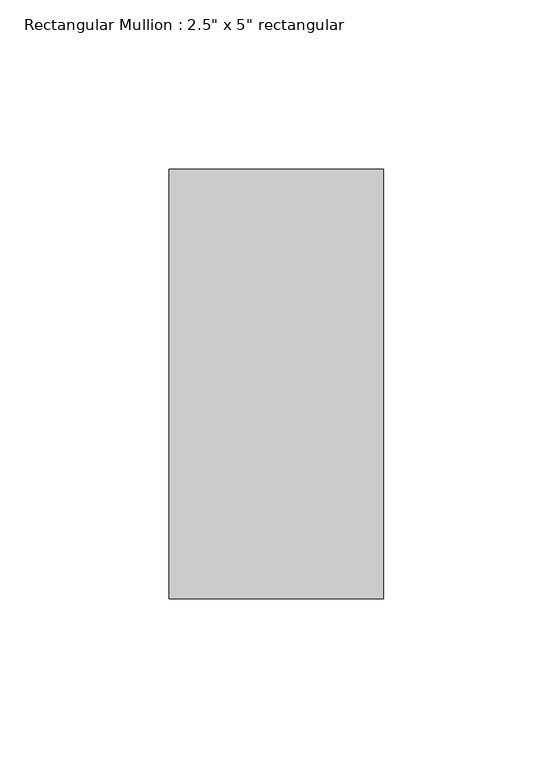
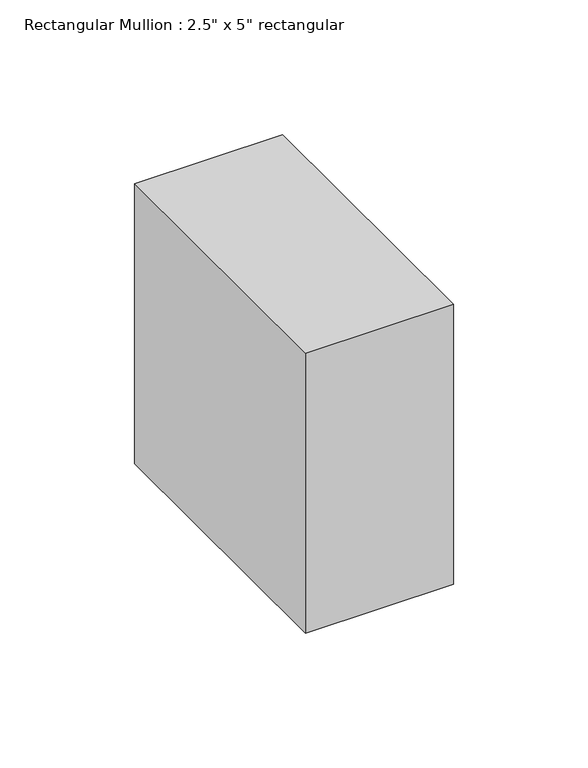
"""IFC4 building model written with IfcOpenShell, lengths in millimetres: member geometry."""

from ifc_helpers import new_model, si_unit, frame, origin, place, context, project, spatial, polyline, outline, extrude, source, transform, mapped, element, save


def member_a8e3eee7(model_context):
    return source(origin(), model_context, "Body", "SweptSolid", [
        extrude(outline(polyline([(0.0, 63.5), (0.0, -63.5), (-63.5, -63.5), (-63.5, 63.5), (0.0, 63.5)])), frame((0.0, 0.0, -127.0), z_axis=(0.0, 0.0, 1.0), x_axis=(1.0, 0.0, 0.0)), (0.0, 0.0, 1.0), 127.0),
    ])


if __name__ == "__main__":
    model = new_model("IFC4")
    model_context = context("Model", 3, world=origin())
    ifc_project = project(units=[si_unit("LENGTHUNIT", "METRE", prefix="MILLI")], contexts=[model_context])
    site = spatial("IfcSite", under=ifc_project)
    building = spatial("IfcBuilding", under=site)
    placement = place(None, origin())
    member_shape = member_a8e3eee7(model_context)
    element("IfcMember", 1, ObjectType="Rectangular Mullion : 2.5\" x 5\" rectangular", at=placement, inside=building, context=model_context, shape_type="MappedRepresentation", body=[
        mapped(member_shape, transform((0.0, 0.0, 0.0), x_axis=(1.0, 0.0, 0.0), y_axis=(0.0, 1.0, 0.0), z_axis=(0.0, 0.0, 1.0))),
    ])
    save(model, "model.ifc")

# Revit data of these elements
# Type "Rectangular Mullion : 2.5\" x 5\" rectangular"
#   built-in parameter 1007304 = 0.416667 (stored number, unit not read)
#   built-in parameter 1007301 = 0.104167 (stored number, unit not read)
#   built-in parameter 1007300 = 0.104167 (stored number, unit not read)
# Element 1 (IfcMember, "Rectangular Mullion : 2.5\" x 5\" rectangular")
#   Materials on its faces: "Door - Frame"
# Materials
#   "Door - Frame": colour RGB 118 70 51, transparency 0, Cost = 0
